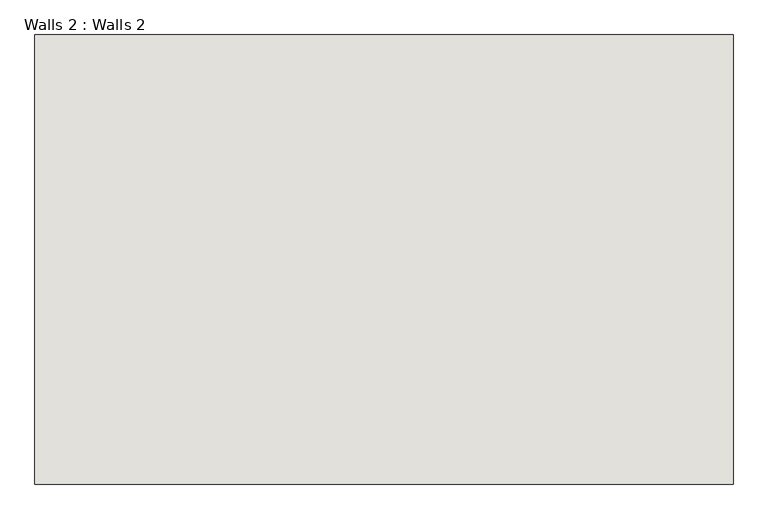
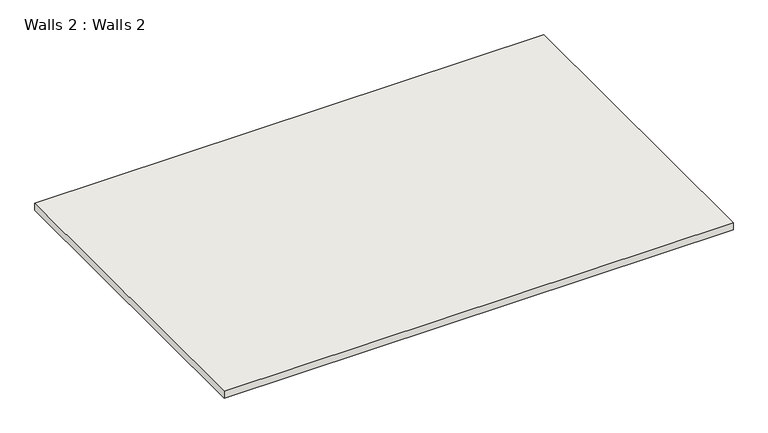
"""IFC4 building model written with IfcOpenShell, lengths in millimetres: wall geometry, Walls 2 : Walls 2."""

from ifc_helpers import new_model, si_unit, frame, origin, place, context, project, spatial, polyline, outline, extrude, source, transform, mapped, element, save


def walls_2_walls_2_982de27e(model_context):
    return source(origin(), model_context, "Body", "SweptSolid", [
        extrude(outline(polyline([(1966.4339443, -13907.4064876), (-19826.7660557, -13907.4064876), (-19826.7660557, 113.3935124), (1966.4339443, 113.3935124), (1966.4339443, -13907.4064876)])), frame((0.0, 0.0, 9144.0), z_axis=(0.0, 0.0, 1.0), x_axis=(1.0, 0.0, 0.0)), (0.0, 0.0, 1.0), 304.8),
    ])


if __name__ == "__main__":
    model = new_model("IFC4")
    model_context = context("Model", 3, world=origin())
    ifc_project = project(units=[si_unit("LENGTHUNIT", "METRE", prefix="MILLI")], contexts=[model_context])
    site = spatial("IfcSite", under=ifc_project)
    building = spatial("IfcBuilding", under=site)
    placement = place(None, origin())
    walls_2_walls_2_shape = walls_2_walls_2_982de27e(model_context)
    element("IfcWall", 1, ObjectType="Walls 2 : Walls 2", at=placement, inside=building, context=model_context, shape_type="MappedRepresentation", body=[
        mapped(walls_2_walls_2_shape, transform((0.0, 0.0, 0.0), x_axis=(1.0, 0.0, 0.0), y_axis=(0.0, 1.0, 0.0), z_axis=(0.0, 0.0, 1.0))),
    ])
    save(model, "model.ifc")

# Revit data of these elements
# Element 1 (IfcWall, "Walls 2 : Walls 2")
#   Materials on its faces: "Default Wall"
# Materials
#   "Default Wall": colour RGB 80 80 80, transparency 0
